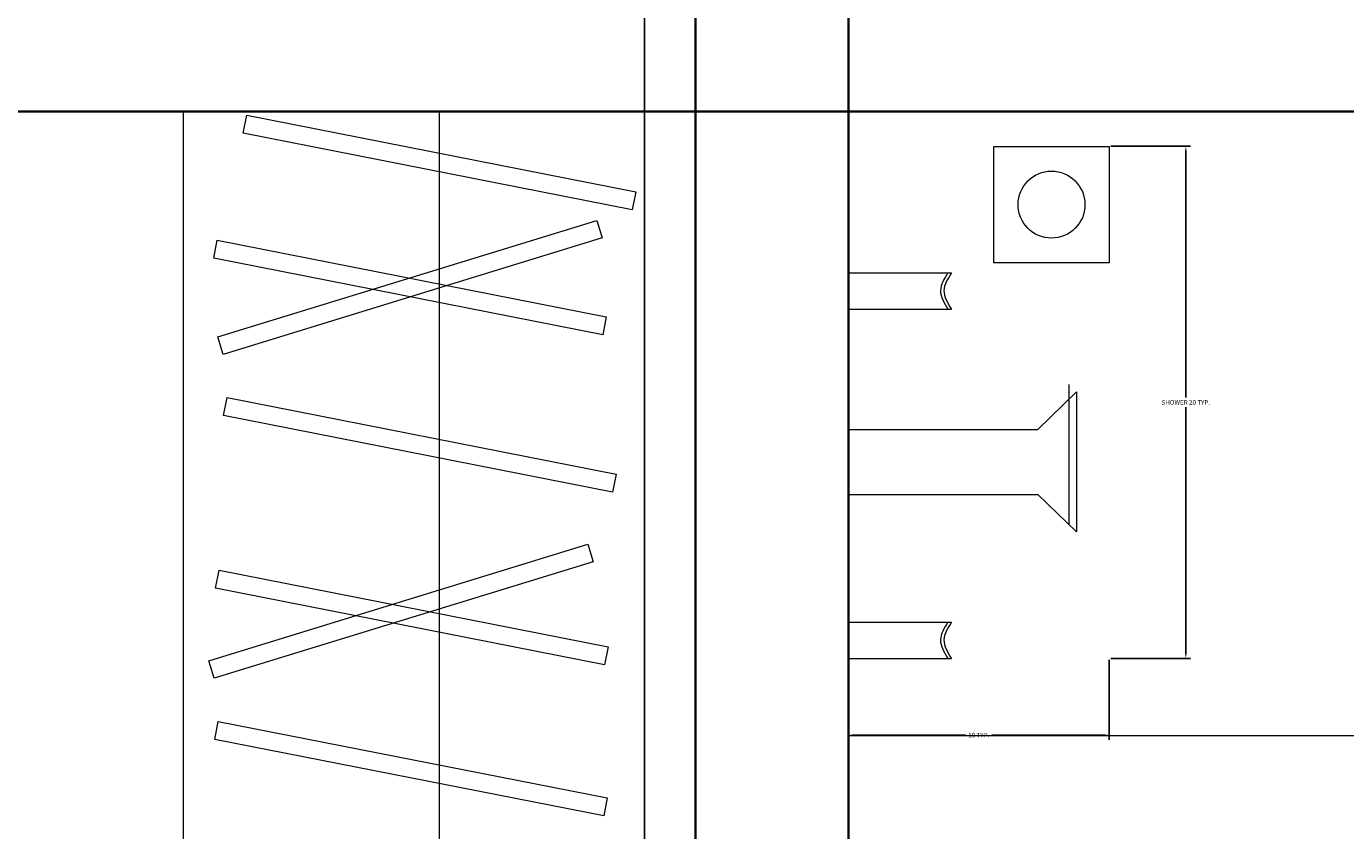
# Model space of a CAD drawing. Units: inches. Extents: x -61 to 1599, y -1316 to 257.
# Tile 70 of 204: x 295 to 347, y -654 to -623. Entities that reach past the tile are written whole.
import ezdxf

# ---------------------------------------------------------------- set-up
doc = ezdxf.new("R2010")
doc.units = ezdxf.units.IN
doc.header["$MEASUREMENT"] = 0
for name, color, linetype, lineweight in [('A-ANNO-DIMS', 2, 'Continuous', 18), ('A-FLOR-CASE', 8, 'Continuous', 18), ('A-FLOR-FIXT', 8, 'Continuous', 18), ('WALLS', 4, 'Continuous', 35)]:
    doc.layers.add(name, color=color, linetype=linetype, lineweight=lineweight)
doc.styles.get("Standard").update_dxf_attribs({"font": 'arial.ttf'})
doc.dimstyles.get("Standard").update_dxf_attribs({"dimtxt": 0.18, "dimasz": 0.18, "dimexe": 0.18, "dimexo": 0.0625, "dimgap": 0.09, "dimtad": 0, "dimtih": 1, "dimtoh": 1, "dimdec": 0, "dimzin": 0, "dimdsep": 46, "dimlunit": 3, "dimtxsty": 'Standard', "dimcen": 0.09, "dimadec": 0, "dimazin": 0, "dimtfac": 1, "dimtdec": 0, "dimtofl": 0, "dimtmove": 0, "dimatfit": 3, "dimfxl": 1, "dimtolj": 1, "dimtzin": 0, "dimarcsym": 0})

# ---------------------------------------------------------------- blocks, each defined once
blk = doc.blocks.new('SHOWER-FITTINGS-2')
for p, q in [((0, 15.11), (4.042, 15.11)), ((0, 13.693), (4.042, 13.693)), ((7.429, 8.977), (8.952, 10.45)), ((8.658, 10.735), (8.658, 5.241)), ((8.952, 10.45), (8.952, 4.957)), ((0, 8.977), (7.429, 8.977)), ((0, 6.429), (7.429, 6.429)), ((7.429, 6.429), (8.952, 4.957)), ((0, 1.417), (4.042, 1.417)), ((0, 0), (4.042, 0))]:
    blk.add_line(p, q)
blk.add_lwpolyline([(10.232, 15.504), (5.711, 15.504), (5.711, 20.076), (10.232, 20.076)], close=True)
blk.add_circle((7.972, 17.79), 1.313)
for points in [[(3.906, 15.11), (3.762, 14.88), (3.468, 14.41), (3.758, 13.935), (3.906, 13.693)], [(4.042, 15.11), (3.898, 14.88), (3.604, 14.41), (3.894, 13.935), (4.042, 13.693)], [(3.906, 1.417), (3.762, 1.187), (3.468, 0.717), (3.758, 0.242), (3.906, 0)], [(4.042, 1.417), (3.898, 1.187), (3.604, 0.717), (3.894, 0.242), (4.042, 0)]]:
    blk.add_open_spline(points, degree=3, knots=[0, 0, 0, 0, 0.7501, 1.532449, 1.532449, 1.532449, 1.532449])
blk = doc.blocks.new('WARDROBE-HANGING')
blk.add_line((10.047, 0), (10.047, 68))
for points in [[(20.094, 0), (0, 0), (0, 68), (20.094, 68)], [(2.482, 67.852), (17.751, 64.849), (17.612, 64.142), (2.343, 67.146)], [(1.346, 59.162), (16.221, 63.731), (16.432, 63.043), (1.557, 58.474)], [(1.325, 62.957), (16.593, 59.954), (16.454, 59.247), (1.186, 62.251)], [(1.713, 56.784), (16.981, 53.781), (16.842, 53.074), (1.574, 56.078)], [(0.997, 46.467), (15.872, 51.036), (16.084, 50.348), (1.209, 45.779)], [(1.394, 50.014), (16.662, 47.011), (16.523, 46.305), (1.255, 49.308)], [(1.365, 44.09), (16.633, 41.086), (16.494, 40.38), (1.226, 43.383)]]:
    blk.add_lwpolyline(points, close=True)
blk = doc.blocks.new('*D652')
at = {"layer": 'A-ANNO-DIMS', "color": 0, "lineweight": -2, "transparency": 16777216}
for p, q in [((337.997, -627.308), (341.126, -627.308)), ((340.946, -627.488), (340.946, -637.163)), ((340.946, -647.205), (340.946, -637.53)), ((337.997, -647.385), (341.126, -647.385))]:
    blk.add_line(p, q, dxfattribs=at)
at = {"layer": 'A-ANNO-DIMS', "color": 0, "transparency": 16777216}
for points in [[(340.916, -627.488), (340.976, -627.488), (340.946, -627.308)], [(340.916, -647.205), (340.976, -647.205), (340.946, -647.385)]]:
    blk.add_solid(points, dxfattribs=at)
at = {"layer": 'DEFPOINTS', "color": 0, "transparency": 16777216}
for p in [(337.935, -627.308), (340.946, -627.308), (337.935, -647.385)]:
    blk.add_point(p, dxfattribs=at)
at = {"layer": 'A-ANNO-DIMS', "color": 0, "transparency": 16777216, "insert": (340.946, -637.347), "char_height": 0.18, "attachment_point": 5}
blk.add_mtext('\\A1;SHOWER 20 TYP.', dxfattribs=at)
blk = doc.blocks.new('*D653')
at = {"layer": 'A-ANNO-DIMS', "color": 0, "lineweight": -2, "transparency": 16777216}
for p, q in [((327.703, -647.447), (327.703, -650.576)), ((337.935, -647.447), (337.935, -650.576)), ((327.883, -650.396), (332.299, -650.396)), ((337.755, -650.396), (333.338, -650.396))]:
    blk.add_line(p, q, dxfattribs=at)
at = {"layer": 'A-ANNO-DIMS', "color": 0, "transparency": 16777216}
for points in [[(327.883, -650.366), (327.883, -650.426), (327.703, -650.396)], [(337.755, -650.366), (337.755, -650.426), (337.935, -650.396)]]:
    blk.add_solid(points, dxfattribs=at)
at = {"layer": 'DEFPOINTS', "color": 0, "transparency": 16777216}
for p in [(327.703, -647.385), (337.935, -647.385), (337.935, -650.396)]:
    blk.add_point(p, dxfattribs=at)
at = {"layer": 'A-ANNO-DIMS', "color": 0, "transparency": 16777216, "insert": (332.819, -650.396), "char_height": 0.18, "attachment_point": 5}
blk.add_mtext('\\A1;10 TYP.', dxfattribs=at)
blk = doc.blocks.new('*D687')
at = {"layer": 'A-ANNO-DIMS', "color": 0, "lineweight": -2, "transparency": 16777216}
for p, q in [((289.418, 181.677), (-61.077, 181.677)), ((-60.897, 181.497), (-60.897, -528.952)), ((-60.897, -1239.765), (-60.897, -529.316)), ((319.64, -1239.945), (-61.077, -1239.945))]:
    blk.add_line(p, q, dxfattribs=at)
at = {"layer": 'A-ANNO-DIMS', "color": 0, "transparency": 16777216}
for points in [[(-60.927, 181.497), (-60.867, 181.497), (-60.897, 181.677)], [(-60.927, -1239.765), (-60.867, -1239.765), (-60.897, -1239.945)]]:
    blk.add_solid(points, dxfattribs=at)
at = {"layer": 'DEFPOINTS', "color": 0, "transparency": 16777216}
for p in [(289.481, 181.677), (-60.897, -1239.945), (319.703, -1239.945)]:
    blk.add_point(p, dxfattribs=at)
at = {"layer": 'A-ANNO-DIMS', "color": 0, "transparency": 16777216, "insert": (-60.897, -529.134), "char_height": 0.18, "attachment_point": 5}
blk.add_mtext('\\A1;1421.6', dxfattribs=at)
blk = doc.blocks.new('*D710')
at = {"layer": 'A-ANNO-DIMS', "color": 0, "lineweight": -2, "transparency": 16777216}
for p, q in [((319.703, -465.385), (319.703, -1315.725)), ((403.703, -465.385), (403.703, -1315.725)), ((319.883, -1315.545), (361.484, -1315.545)), ((403.523, -1315.545), (361.921, -1315.545))]:
    blk.add_line(p, q, dxfattribs=at)
at = {"layer": 'A-ANNO-DIMS', "color": 0, "transparency": 16777216}
for points in [[(319.883, -1315.515), (319.883, -1315.575), (319.703, -1315.545)], [(403.523, -1315.515), (403.523, -1315.575), (403.703, -1315.545)]]:
    blk.add_solid(points, dxfattribs=at)
at = {"layer": 'DEFPOINTS', "color": 0, "transparency": 16777216}
for p in [(319.703, -465.323), (403.703, -465.323), (403.703, -1315.545)]:
    blk.add_point(p, dxfattribs=at)
at = {"layer": 'A-ANNO-DIMS', "color": 0, "transparency": 16777216, "insert": (361.703, -1315.545), "char_height": 0.18, "attachment_point": 5}
blk.add_mtext('\\A1;84', dxfattribs=at)

msp = doc.modelspace()

# ---------------------------------------------------------------- linework, layer by layer
at = {"layer": 'A-FLOR-FIXT'}
msp.add_line((327.7028, -650.414), (397.7028, -650.414), dxfattribs=at)
at = {"layer": 'WALLS'}
for p, q in [((321.7028, -616.9446), (321.7028, -787.9446)), ((327.7028, -616.9446), (327.7028, -787.9446)), ((237.7028, -625.9446), (321.7028, -625.9446)), ((321.7028, -625.9446), (327.7028, -625.9446)), ((327.7028, -625.9446), (397.7028, -625.9446))]:
    msp.add_line(p, q, dxfattribs=at)

# ---------------------------------------------------------------- block references
at = {"layer": 'A-FLOR-CASE'}
msp.add_blockref('WARDROBE-HANGING', (301.609, -693.9447), dxfattribs=at)
at = {"layer": 'A-FLOR-FIXT'}
msp.add_blockref('SHOWER-FITTINGS-2', (327.703, -647.3847), dxfattribs=at)

# ---------------------------------------------------------------- dimensions: what is measured, and where the dimension line sits
at = {"layer": 'A-ANNO-DIMS'}
dim = msp.add_linear_dim(base=(-60.8972, -1239.9446), p1=(289.4807, 181.6771), p2=(319.7028, -1239.9446), angle=90, dimstyle='Standard', override={"dimdec": 1, "dimlfac": 1, "dimrnd": 0, "dimzin": 0, "dimdsep": 46, "dimlunit": 2}, dxfattribs=at)
dim.commit()
dim.dimension.update_dxf_attribs({"geometry": '*D687', "text_midpoint": (-60.8972, -529.1337)})
dim = msp.add_linear_dim(base=(403.7028, -1315.5446), p1=(319.7028, -465.3229), p2=(403.7028, -465.3229), dimstyle='Standard', override={"dimdec": 0, "dimlfac": 1, "dimrnd": 0, "dimzin": 0, "dimdsep": 46, "dimlunit": 2}, dxfattribs=at)
dim.commit()
dim.dimension.update_dxf_attribs({"geometry": '*D710', "text_midpoint": (361.7028, -1315.5446)})
dim = msp.add_linear_dim(base=(340.9463, -627.3082), p1=(337.9348, -647.3849), p2=(337.9348, -627.3082), angle=90, text='SHOWER <> TYP.', dimstyle='Standard', override={"dimdec": 0, "dimlfac": 1, "dimrnd": 0, "dimzin": 0, "dimdsep": 46, "dimlunit": 2}, dxfattribs=at)
dim.commit()
dim.dimension.update_dxf_attribs({"geometry": '*D652', "text_midpoint": (340.9463, -637.3466)})
dim = msp.add_linear_dim(base=(337.9348, -650.3965), p1=(327.7028, -647.3849), p2=(337.9348, -647.3849), text='<> TYP.', dimstyle='Standard', override={"dimdec": 0, "dimlfac": 1, "dimrnd": 0, "dimzin": 0, "dimdsep": 46, "dimlunit": 2}, dxfattribs=at)
dim.commit()
dim.dimension.update_dxf_attribs({"geometry": '*D653', "text_midpoint": (332.8188, -650.3965)})

doc.saveas('drawing.dxf')
